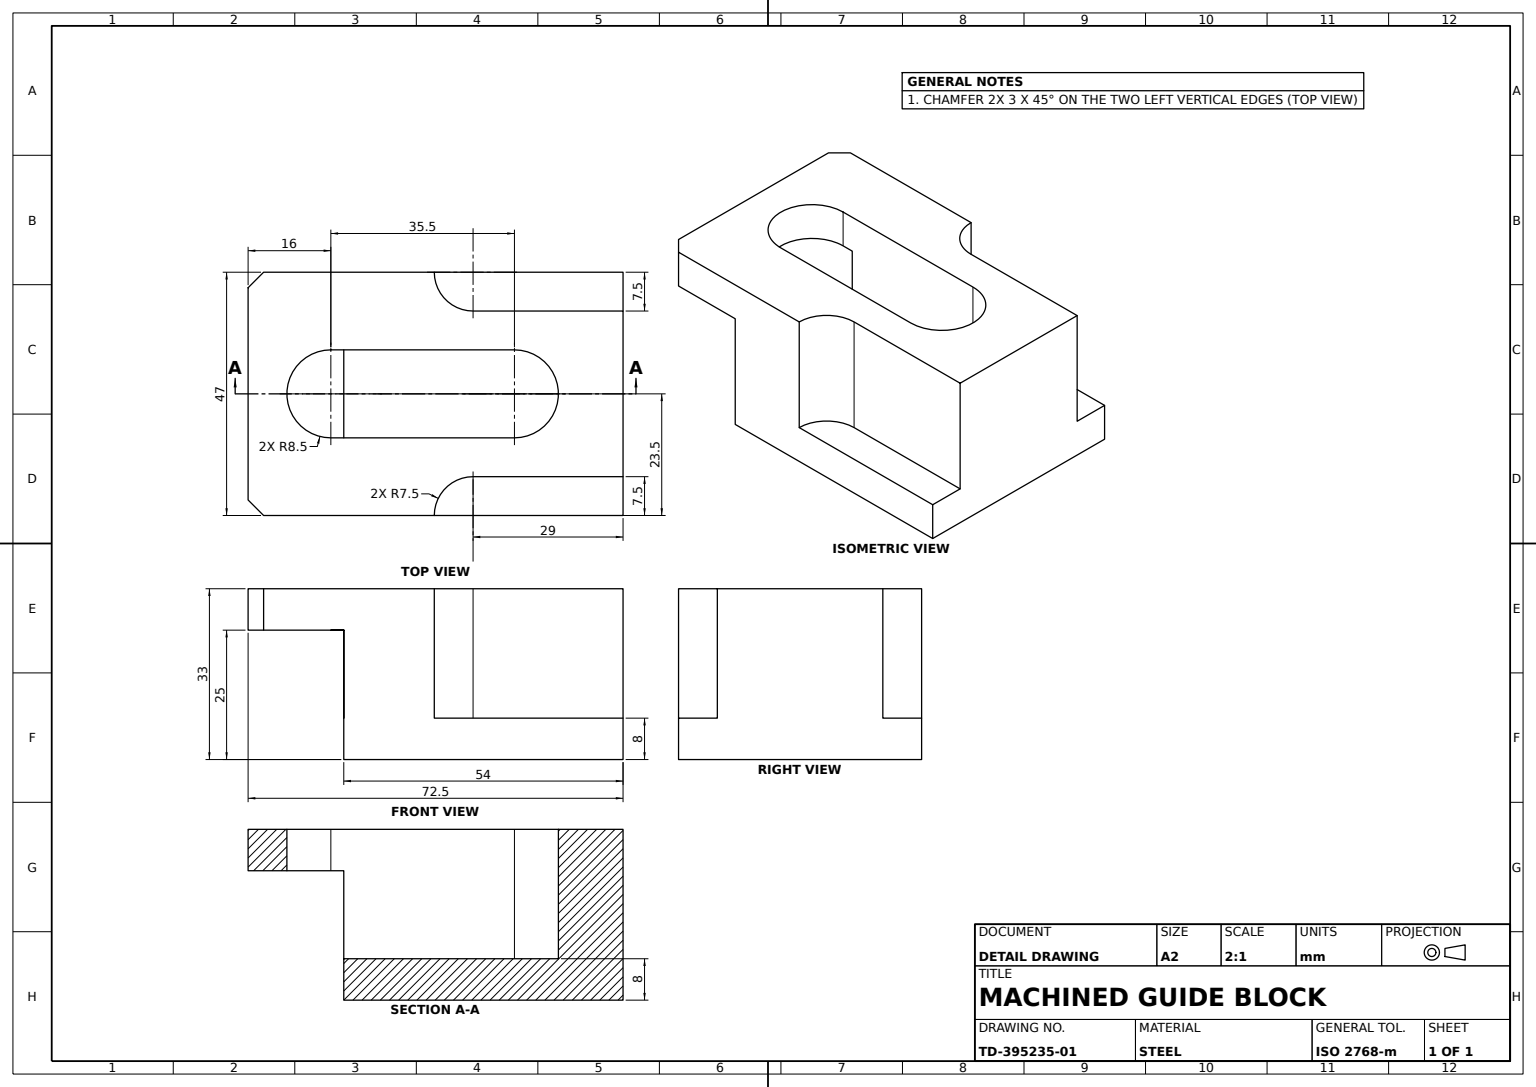
SolidWorks part; units mm, degrees
material "Plain Carbon Steel"
ref_plane "Front Plane" through (0, 0, 0) normal (0, 0, 1) x (1, 0, 0)
ref_plane "Top Plane" through (0, 0, 0) normal (0, 1, 0) x (1, 0, 0)
ref_plane "Right Plane" through (0, 0, 0) normal (1, 0, 0) x (0, 0, -1)
sketch "Base Profile Sketch" plane through (0, 0, 0) normal (0, 0, 1) x (1, 0, 0)
  line L0 (0, 0) -> (54, 0)
  line L1 (54, 0) -> (54, 8)
  line L5 (-18.5, 33) -> (-18.5, 25)
  line L6 (-18.5, 25) -> (0, 25)
  line L7 (0, 25) -> (0, 0)
  line L8 (54, 8) -> (54, 33)
  line L9 (54, 33) -> (-18.5, 33)
  dimension "D1" = 54
  dimension "D2" = 8
  dimension "D3" = 25
  dimension "D4" = 72.5
  dimension "D5" = 8
extrude "Base Block" add sketch "Base Profile Sketch" against normal blind 47
sketch "Side Notch A Sketch" plane through (0, 33, 0) normal (0, 1, 0) x (1, 0, 0)
  line L0 (54, 0) -> (54, 7.5)
  line L1 (54, 47) -> (54, 0) construction
  line L2 (54, 7.5) -> (25, 7.5)
  line L4 (54, 0) -> (-18.5, 0) construction
  line L6 (25, 0) -> (17.5, 0)
  line L7 (25, 0) -> (54, 0)
  arc A0 (25, 7.5) -> (17.5, 0) centre (25, 0) ccw
  dimension "D1" = 7.5
  dimension "D2" = 29
extrude "Side Notch A" cut sketch "Side Notch A Sketch" against normal blind 25
sketch "Side Notch B Sketch" plane through (0, 33, 0) normal (0, 1, 0) x (1, 0, 0)
  line L0 (54, 47) -> (54, 39.5)
  line L1 (54, 47) -> (54, 7.5) construction
  line L2 (54, 39.5) -> (25, 39.5)
  line L4 (54, 47) -> (-18.5, 47) construction
  line L5 (25, 47) -> (54, 47)
  line L6 (17.5, 47) -> (25, 47)
  arc A0 (17.5, 47) -> (25, 39.5) centre (25, 47) ccw
  arc A1 (25, 7.5) -> (17.5, 0) centre (25, 0) ccw construction
  dimension "D1" = 7.5
  dimension "D2" = 29
extrude "Side Notch B" cut sketch "Side Notch B Sketch" against normal blind 25
sketch "Guide Slot Sketch" plane through (0, 33, 0) normal (0, 1, 0) x (1, 0, 0)
  line L0 (-2.5, 23.5) -> (33, 23.5) construction
  line L1 (-2.5, 32) -> (33, 32)
  line L2 (-2.5, 15) -> (33, 15)
  line L3 (17.5, 0) -> (-18.5, 0) construction
  line L5 (-18.5, 47) -> (-18.5, 0) construction
  arc A0 (-2.5, 32) -> (-2.5, 15) centre (-2.5, 23.5) ccw
  arc A1 (33, 15) -> (33, 32) centre (33, 23.5) ccw
  point P2 (15.25, 23.5)
  dimension "D2" = 8.5
  dimension "D1" = 35.5
  dimension "D3" = 23.5
  dimension "D4" = 16
extrude "Guide Slot" cut sketch "Guide Slot Sketch" against normal blind 25
chamfer "Edge Chamfer 3x45" distance 3 angle 45 2 edges at (-18.5, 29, -47) (-18.5, 29, 0)
